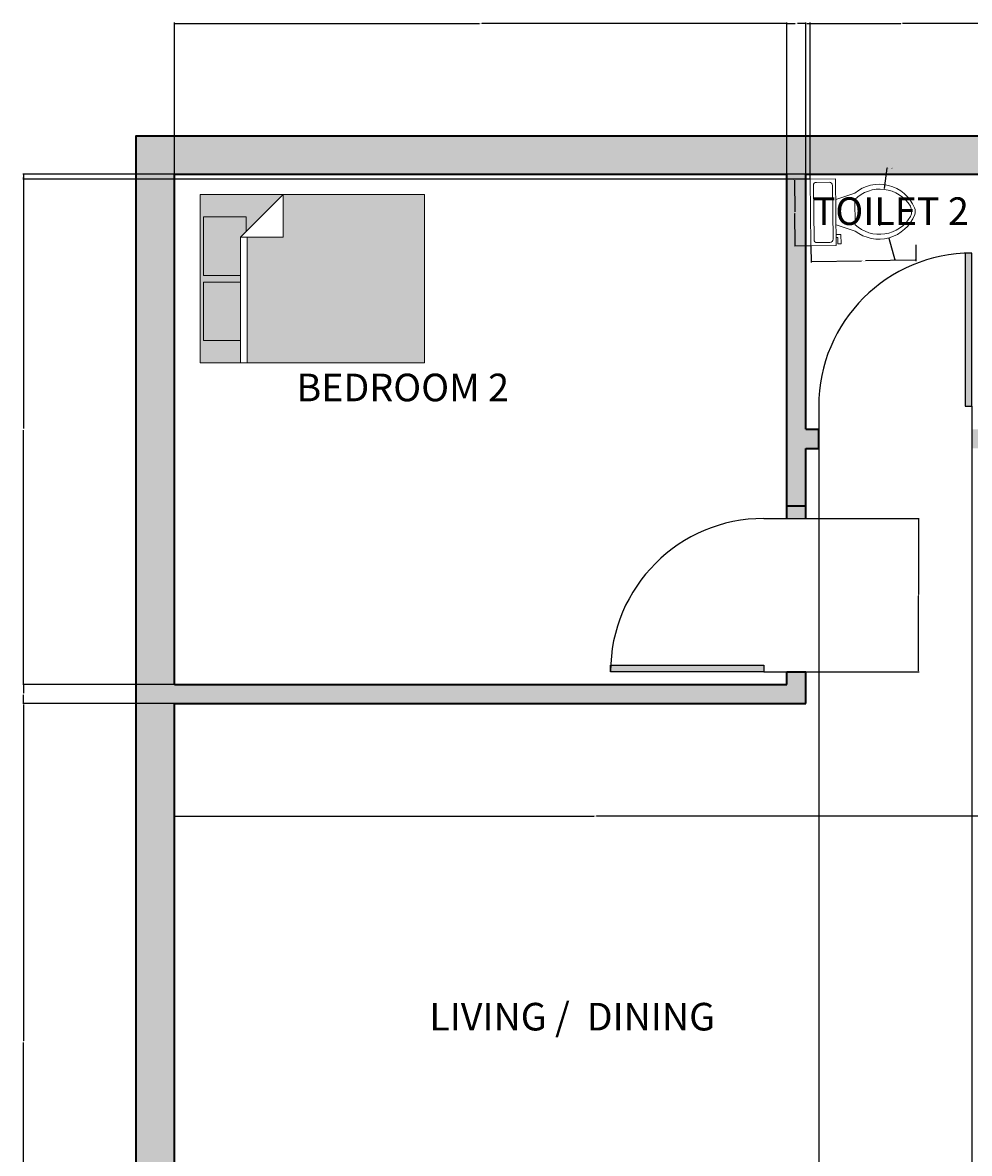
# Model space of a CAD drawing. Units: inches. Extents: x 1034 to 1730, y 674 to 1249.
# Tile 3 of 4: x 1316 to 1538, y 983 to 1249. Entities that reach past the tile are written whole.
import ezdxf

# ---------------------------------------------------------------- set-up
doc = ezdxf.new("R2010")
doc.units = ezdxf.units.IN
for name, color, linetype, lineweight in [('A-ANNO-DIMS', 2, 'Continuous', 18), ('A-AREA-IDEN', 7, 'Continuous', 18), ('A-DOOR', 4, 'Continuous', 25), ('A-FLOR-FIXT', 9, 'Continuous', 18), ('A-FURN', 9, 'Continuous', 18), ('A-FURN-PATT', 7, 'Continuous', 13), ('A-WALL', 7, 'Continuous', 35), ('A-WALL-PATT', 8, 'Continuous', 13)]:
    doc.layers.add(name, color=color, linetype=linetype, lineweight=lineweight)
doc.layers.add('A-DOOR-PATT', color=17, linetype='Continuous', lineweight=13, true_color=0x7b4636)
doc.styles.get("Standard").update_dxf_attribs({"font": 'arial.ttf'})
doc.dimstyles.get("Standard").update_dxf_attribs({"dimtxt": 0.18, "dimasz": 0.18, "dimexe": 0.18, "dimexo": 0.0625, "dimgap": 0.09, "dimtad": 0, "dimtih": 1, "dimtoh": 1, "dimdec": 4, "dimzin": 0, "dimdsep": 46, "dimtxsty": 'Standard', "dimcen": 0.09, "dimadec": 0, "dimazin": 0, "dimtfac": 1, "dimtdec": 4, "dimtofl": 0, "dimtmove": 0, "dimatfit": 3, "dimfxl": 1, "dimtolj": 1, "dimtzin": 0, "dimarcsym": 0})

# ---------------------------------------------------------------- blocks, each defined once
blk = doc.blocks.new('*U3')
for p, q in [((0, 0), (0, -6)), ((40, 0), (40, -6))]:
    blk.add_line(p, q)
blk.add_lwpolyline([(0, 0), (0, 40), (1.75, 40), (1.75, 0)], close=True)
blk.add_arc((0, 0), 40, 0, 90)
blk = doc.blocks.new('*U5')
for p, q in [((0, 0), (0, -6)), ((-40, 0), (-40, -6))]:
    blk.add_line(p, q)
blk.add_lwpolyline([(0, 0), (0, 40), (-1.75, 40), (-1.75, 0)], close=True)
blk.add_arc((0, 0), 40, 90, 180)
blk = doc.blocks.new('Bed - Queen')
for p, q in [((0, -80.00003), (0, 0)), ((0, 0), (59.99999, 0)), ((59.99999, 0), (59.99999, -80.00003)), ((7.99999, -1.2), (28.79998, -1.2)), ((7.99999, -14.4), (7.99999, -1.2)), ((28.79998, -1.2), (28.79998, -14.4)), ((31.19999, -1.2), (51.99999, -1.2)), ((31.19999, -14.4), (31.19999, -1.2)), ((51.99999, -1.2), (51.99999, -16.4)), ((0, -14.4), (44.8, -14.4)), ((59.99999, -29.6), (44.8, -14.4)), ((44.8, -14.4), (44.8, -29.6)), ((44.8, -16.8), (0, -16.8)), ((51.99999, -16.4), (46.79936, -16.4)), ((44.8, -29.6), (59.99999, -29.6)), ((59.99999, -80.00003), (0, -80.00003))]:
    blk.add_line(p, q)
blk = doc.blocks.new('Toilet - top')
for p, q in [((9.5, -6), (9.5, -2)), ((-10, -8.5), (-8, -8.5)), ((-10, -9.5), (-10, -8.5)), ((-7, -9.5), (-10, -9.5)), ((-8, -8.5), (-8, -8)), ((-7, -8), (-7, -9.5)), ((-4, -8), (-6, -14)), ((4, -8), (6, -14)), ((4, -14), (-4, -14))]:
    blk.add_line(p, q)
blk.add_lwpolyline([(10.5, -8), (10.5, 0), (-10.5, 0), (-10.5, -8)], close=True)
for points in [[(-9.5, -2), (-9.5, -6)], [(8.5, -1), (-8.5, -1)], [(-8.5, -7), (8.5, -7)]]:
    blk.add_lwpolyline(points)
for centre, radius, start, end in [((-8.62, -1.88), 0.884, 81.8699, 188.1301), ((8.62, -1.88), 0.884, 351.8699, 98.1301), ((-8.62, -6.12), 0.884, 171.8699, 278.1301), ((8.62, -6.12), 0.884, 261.8699, 8.1301), ((3.52, -21.58), 12.17, 141.4691, 247.9714), ((4.2, -21.82), 11.33, 136.3677, 238.9468), ((-3.52, -21.58), 12.17, 292.0284, 38.5307), ((-4.2, -21.82), 11.33, 301.053, 43.6321), ((0, -27.88), 4, 245.7318, 294.2682), ((0, -29), 4, 254.8605, 285.1395)]:
    blk.add_arc(centre, radius, start, end)
blk = doc.blocks.new('*D12')
at = {"layer": 'A-ANNO-DIMS', "color": 0, "lineweight": -2, "transparency": 16777216}
for p, q in [((1501.21, 1196.5), (1501.26, 1192.69)), ((1525.84, 1196.81), (1525.89, 1193)), ((1501.43, 1192.87), (1513.1, 1193.02)), ((1525.7, 1193.17), (1514.04, 1193.03))]:
    blk.add_line(p, q, dxfattribs=at)
at = {"layer": 'A-ANNO-DIMS', "color": 0, "transparency": 16777216}
for points in [[(1501.43, 1192.9), (1501.43, 1192.84), (1501.25, 1192.87)], [(1525.7, 1193.2), (1525.7, 1193.14), (1525.88, 1193.18)]]:
    blk.add_solid(points, dxfattribs=at)
at = {"layer": 'Defpoints', "color": 0, "transparency": 16777216}
for p in [(1501.21, 1196.57), (1525.84, 1196.87), (1501.25, 1192.87)]:
    blk.add_point(p, dxfattribs=at)
at = {"layer": 'A-ANNO-DIMS', "color": 0, "transparency": 16777216, "insert": (1513.57, 1193.02), "char_height": 0.18, "attachment_point": 5}
blk.add_mtext('\\A1;WC 25', dxfattribs=at)
blk = doc.blocks.new('*D13')
at = {"layer": 'A-ANNO-DIMS', "color": 0, "lineweight": -2, "transparency": 16777216}
for p, q in [((1500.95, 1212.22), (1497.14, 1212.17)), ((1497.32, 1211.99), (1497.41, 1204.53)), ((1497.51, 1196.7), (1497.42, 1204.16)), ((1501.15, 1196.56), (1497.33, 1196.52))]:
    blk.add_line(p, q, dxfattribs=at)
at = {"layer": 'A-ANNO-DIMS', "color": 0, "transparency": 16777216}
for points in [[(1497.35, 1211.99), (1497.29, 1211.99), (1497.32, 1212.17)], [(1497.54, 1196.7), (1497.48, 1196.7), (1497.51, 1196.52)]]:
    blk.add_solid(points, dxfattribs=at)
at = {"layer": 'Defpoints', "color": 0, "transparency": 16777216}
for p in [(1497.32, 1212.17), (1501.01, 1212.22), (1501.21, 1196.57)]:
    blk.add_point(p, dxfattribs=at)
at = {"layer": 'A-ANNO-DIMS', "color": 0, "transparency": 16777216, "insert": (1497.42, 1204.34), "char_height": 0.18, "attachment_point": 5}
blk.add_mtext('\\A1;16', dxfattribs=at)
blk = doc.blocks.new('*D17')
at = {"layer": 'A-ANNO-DIMS', "color": 0, "lineweight": -2, "transparency": 16777216}
for p, q in [((1351.53, 1213.49), (1351.53, 1249.06)), ((1351.71, 1248.88), (1423.25, 1248.88)), ((1495.35, 1248.88), (1423.81, 1248.88)), ((1495.53, 1213.49), (1495.53, 1249.06))]:
    blk.add_line(p, q, dxfattribs=at)
at = {"layer": 'A-ANNO-DIMS', "color": 0, "transparency": 16777216}
for points in [[(1351.71, 1248.91), (1351.71, 1248.85), (1351.53, 1248.88)], [(1495.35, 1248.91), (1495.35, 1248.85), (1495.53, 1248.88)]]:
    blk.add_solid(points, dxfattribs=at)
at = {"layer": 'Defpoints', "color": 0, "transparency": 16777216}
for p in [(1495.53, 1248.88), (1351.53, 1213.43), (1495.53, 1213.43)]:
    blk.add_point(p, dxfattribs=at)
at = {"layer": 'A-ANNO-DIMS', "color": 0, "transparency": 16777216, "insert": (1423.53, 1248.88), "char_height": 0.18, "attachment_point": 5}
blk.add_mtext('\\A1;144', dxfattribs=at)
blk = doc.blocks.new('*D19')
at = {"layer": 'A-ANNO-DIMS', "color": 0, "lineweight": -2, "transparency": 16777216}
for p, q in [((1351.47, 1213.43), (1315.9, 1213.43)), ((1316.08, 1213.25), (1316.08, 1153.61)), ((1316.08, 1093.61), (1316.08, 1153.24)), ((1351.47, 1093.43), (1315.9, 1093.43))]:
    blk.add_line(p, q, dxfattribs=at)
at = {"layer": 'A-ANNO-DIMS', "color": 0, "transparency": 16777216}
for points in [[(1316.05, 1213.25), (1316.11, 1213.25), (1316.08, 1213.43)], [(1316.05, 1093.61), (1316.11, 1093.61), (1316.08, 1093.43)]]:
    blk.add_solid(points, dxfattribs=at)
at = {"layer": 'Defpoints', "color": 0, "transparency": 16777216}
for p in [(1316.08, 1213.43), (1351.53, 1213.43), (1351.53, 1093.43)]:
    blk.add_point(p, dxfattribs=at)
at = {"layer": 'A-ANNO-DIMS', "color": 0, "transparency": 16777216, "insert": (1316.08, 1153.43), "char_height": 0.18, "attachment_point": 5}
blk.add_mtext('\\A1;120', dxfattribs=at)
blk = doc.blocks.new('*D20')
at = {"layer": 'A-ANNO-DIMS', "color": 0, "lineweight": -2, "transparency": 16777216}
for p, q in [((1351.47, 1088.93), (1315.9, 1088.93)), ((1316.08, 1088.75), (1316.08, 1009.61)), ((1316.08, 930.11), (1316.08, 1009.24)), ((1351.47, 929.93), (1315.9, 929.93))]:
    blk.add_line(p, q, dxfattribs=at)
at = {"layer": 'A-ANNO-DIMS', "color": 0, "transparency": 16777216}
for points in [[(1316.05, 1088.75), (1316.11, 1088.75), (1316.08, 1088.93)], [(1316.05, 930.11), (1316.11, 930.11), (1316.08, 929.93)]]:
    blk.add_solid(points, dxfattribs=at)
at = {"layer": 'Defpoints', "color": 0, "transparency": 16777216}
for p in [(1316.08, 1088.93), (1351.53, 1088.93), (1351.53, 929.93)]:
    blk.add_point(p, dxfattribs=at)
at = {"layer": 'A-ANNO-DIMS', "color": 0, "transparency": 16777216, "insert": (1316.08, 1009.43), "char_height": 0.18, "attachment_point": 5}
blk.add_mtext('\\A1;159', dxfattribs=at)
blk = doc.blocks.new('*D26')
at = {"layer": 'A-ANNO-DIMS', "color": 0, "lineweight": -2, "transparency": 16777216}
for p, q in [((1500.03, 1213.49), (1500.03, 1249.06)), ((1500.21, 1248.88), (1522.31, 1248.88)), ((1544.85, 1248.88), (1522.75, 1248.88)), ((1545.03, 1213.49), (1545.03, 1249.06))]:
    blk.add_line(p, q, dxfattribs=at)
at = {"layer": 'A-ANNO-DIMS', "color": 0, "transparency": 16777216}
for points in [[(1500.21, 1248.91), (1500.21, 1248.85), (1500.03, 1248.88)], [(1544.85, 1248.91), (1544.85, 1248.85), (1545.03, 1248.88)]]:
    blk.add_solid(points, dxfattribs=at)
at = {"layer": 'Defpoints', "color": 0, "transparency": 16777216}
for p in [(1545.03, 1248.88), (1500.03, 1213.43), (1545.03, 1213.43)]:
    blk.add_point(p, dxfattribs=at)
at = {"layer": 'A-ANNO-DIMS', "color": 0, "transparency": 16777216, "insert": (1522.53, 1248.88), "char_height": 0.18, "attachment_point": 5}
blk.add_mtext('\\A1;45', dxfattribs=at)
blk = doc.blocks.new('*D28')
at = {"layer": 'A-ANNO-DIMS', "color": 0, "lineweight": -2, "transparency": 16777216}
for p, q in [((1503.03, 1153.36), (1503.03, 673.53)), ((1539.03, 1153.36), (1539.03, 673.53)), ((1503.21, 673.71), (1520.81, 673.71)), ((1538.85, 673.71), (1521.25, 673.71))]:
    blk.add_line(p, q, dxfattribs=at)
at = {"layer": 'A-ANNO-DIMS', "color": 0, "transparency": 16777216}
for points in [[(1503.21, 673.74), (1503.21, 673.68), (1503.03, 673.71)], [(1538.85, 673.74), (1538.85, 673.68), (1539.03, 673.71)]]:
    blk.add_solid(points, dxfattribs=at)
at = {"layer": 'Defpoints', "color": 0, "transparency": 16777216}
for p in [(1503.03, 1153.43), (1539.03, 1153.43), (1539.03, 673.71)]:
    blk.add_point(p, dxfattribs=at)
at = {"layer": 'A-ANNO-DIMS', "color": 0, "transparency": 16777216, "insert": (1521.03, 673.71), "char_height": 0.18, "attachment_point": 5}
blk.add_mtext('\\A1;36', dxfattribs=at)
blk = doc.blocks.new('*D43')
at = {"layer": 'A-ANNO-DIMS', "color": 0, "lineweight": -2, "transparency": 16777216}
for p, q in [((1495.53, 1213.49), (1495.53, 1249.06)), ((1495.71, 1248.88), (1497.52, 1248.88)), ((1499.85, 1248.88), (1498.04, 1248.88)), ((1500.03, 1213.49), (1500.03, 1249.06))]:
    blk.add_line(p, q, dxfattribs=at)
at = {"layer": 'A-ANNO-DIMS', "color": 0, "transparency": 16777216}
for points in [[(1495.71, 1248.91), (1495.71, 1248.85), (1495.53, 1248.88)], [(1499.85, 1248.91), (1499.85, 1248.85), (1500.03, 1248.88)]]:
    blk.add_solid(points, dxfattribs=at)
at = {"layer": 'Defpoints', "color": 0, "transparency": 16777216}
for p in [(1500.03, 1248.88), (1495.53, 1213.43), (1500.03, 1213.43)]:
    blk.add_point(p, dxfattribs=at)
at = {"layer": 'A-ANNO-DIMS', "color": 0, "transparency": 16777216, "insert": (1497.78, 1248.88), "char_height": 0.18, "attachment_point": 5}
blk.add_mtext('\\A1;4.5', dxfattribs=at)
blk = doc.blocks.new('*D45')
at = {"layer": 'A-ANNO-DIMS', "color": 0, "lineweight": -2, "transparency": 16777216}
for p, q in [((1500.09, 1132.43), (1526.66, 1132.43)), ((1526.48, 1132.25), (1526.48, 1114.61)), ((1526.48, 1096.61), (1526.48, 1114.24)), ((1500.09, 1096.43), (1526.66, 1096.43))]:
    blk.add_line(p, q, dxfattribs=at)
at = {"layer": 'A-ANNO-DIMS', "color": 0, "transparency": 16777216}
for points in [[(1526.45, 1132.25), (1526.51, 1132.25), (1526.48, 1132.43)], [(1526.45, 1096.61), (1526.51, 1096.61), (1526.48, 1096.43)]]:
    blk.add_solid(points, dxfattribs=at)
at = {"layer": 'Defpoints', "color": 0, "transparency": 16777216}
for p in [(1500.03, 1132.43), (1500.03, 1096.43), (1526.48, 1096.43)]:
    blk.add_point(p, dxfattribs=at)
at = {"layer": 'A-ANNO-DIMS', "color": 0, "transparency": 16777216, "insert": (1526.48, 1114.43), "char_height": 0.18, "attachment_point": 5}
blk.add_mtext('\\A1;36', dxfattribs=at)
blk = doc.blocks.new('*D46')
at = {"layer": 'A-ANNO-DIMS', "color": 0, "lineweight": -2, "transparency": 16777216}
for p, q in [((1351.53, 1088.86), (1351.53, 1062.3)), ((1549.53, 1088.86), (1549.53, 1062.3)), ((1351.71, 1062.48), (1450.25, 1062.48)), ((1549.35, 1062.48), (1450.81, 1062.48))]:
    blk.add_line(p, q, dxfattribs=at)
at = {"layer": 'A-ANNO-DIMS', "color": 0, "transparency": 16777216}
for points in [[(1351.71, 1062.51), (1351.71, 1062.45), (1351.53, 1062.48)], [(1549.35, 1062.51), (1549.35, 1062.45), (1549.53, 1062.48)]]:
    blk.add_solid(points, dxfattribs=at)
at = {"layer": 'Defpoints', "color": 0, "transparency": 16777216}
for p in [(1351.53, 1088.93), (1549.53, 1088.93), (1351.53, 1062.48)]:
    blk.add_point(p, dxfattribs=at)
at = {"layer": 'A-ANNO-DIMS', "color": 0, "transparency": 16777216, "insert": (1450.53, 1062.48), "char_height": 0.18, "attachment_point": 5}
blk.add_mtext('\\A1;198', dxfattribs=at)
blk = doc.blocks.new('*D51')
at = {"layer": 'A-ANNO-DIMS', "color": 0, "lineweight": -2, "transparency": 16777216}
for p, q in [((1499.848848, 1248.87622), (1499.668848, 1248.87622)), ((1500.028848, 1213.48872), (1500.028848, 1249.05622)), ((1501.01344, 1212.278928), (1501.01344, 1249.05622)), ((1501.19344, 1248.87622), (1501.37344, 1248.87622))]:
    blk.add_line(p, q, dxfattribs=at)
at = {"layer": 'A-ANNO-DIMS', "color": 0, "transparency": 16777216}
for points in [[(1499.848848, 1248.90622), (1499.848848, 1248.84622), (1500.028848, 1248.87622)], [(1501.19344, 1248.90622), (1501.19344, 1248.84622), (1501.01344, 1248.87622)]]:
    blk.add_solid(points, dxfattribs=at)
at = {"layer": 'Defpoints', "color": 0, "transparency": 16777216}
for p in [(1500.028848, 1248.87622), (1500.028848, 1213.42622), (1501.01344, 1212.216428)]:
    blk.add_point(p, dxfattribs=at)
at = {"layer": 'A-ANNO-DIMS', "color": 0, "transparency": 16777216, "insert": (1500.521144, 1248.87622), "char_height": 0.18, "attachment_point": 5}
blk.add_mtext('\\A1;0.98', dxfattribs=at)
blk = doc.blocks.new('*D52')
at = {"layer": 'A-ANNO-DIMS', "color": 0, "lineweight": -2, "transparency": 16777216}
for p, q in [((1499.97, 1213.43), (1315.9, 1213.43)), ((1316.08, 1213.25), (1316.08, 1213)), ((1316.08, 1212.4), (1316.08, 1212.64)), ((1500.95, 1212.22), (1315.9, 1212.22))]:
    blk.add_line(p, q, dxfattribs=at)
at = {"layer": 'A-ANNO-DIMS', "color": 0, "transparency": 16777216}
for points in [[(1316.05, 1213.25), (1316.11, 1213.25), (1316.08, 1213.43)], [(1316.05, 1212.4), (1316.11, 1212.4), (1316.08, 1212.22)]]:
    blk.add_solid(points, dxfattribs=at)
at = {"layer": 'Defpoints', "color": 0, "transparency": 16777216}
for p in [(1316.08, 1213.43), (1500.03, 1213.43), (1501.01, 1212.22)]:
    blk.add_point(p, dxfattribs=at)
at = {"layer": 'A-ANNO-DIMS', "color": 0, "transparency": 16777216, "insert": (1316.08, 1212.82), "char_height": 0.18, "attachment_point": 5}
blk.add_mtext('\\A1;1.21', dxfattribs=at)
blk = doc.blocks.new('*D53')
at = {"layer": 'A-ANNO-DIMS', "color": 0, "lineweight": -2, "transparency": 16777216}
for p, q in [((1351.47, 1093.43), (1315.9, 1093.43)), ((1316.08, 1093.25), (1316.08, 1091.36)), ((1316.08, 1089.11), (1316.08, 1090.99)), ((1351.47, 1088.93), (1315.9, 1088.93))]:
    blk.add_line(p, q, dxfattribs=at)
at = {"layer": 'A-ANNO-DIMS', "color": 0, "transparency": 16777216}
for points in [[(1316.05, 1093.25), (1316.11, 1093.25), (1316.08, 1093.43)], [(1316.05, 1089.11), (1316.11, 1089.11), (1316.08, 1088.93)]]:
    blk.add_solid(points, dxfattribs=at)
at = {"layer": 'Defpoints', "color": 0, "transparency": 16777216}
for p in [(1316.08, 1093.43), (1351.53, 1093.43), (1351.53, 1088.93)]:
    blk.add_point(p, dxfattribs=at)
at = {"layer": 'A-ANNO-DIMS', "color": 0, "transparency": 16777216, "insert": (1316.08, 1091.18), "char_height": 0.18, "attachment_point": 5}
blk.add_mtext('\\A1;4.5', dxfattribs=at)
blk = doc.blocks.new('*D57')
at = {"layer": 'A-ANNO-DIMS', "color": 0, "lineweight": -2, "transparency": 16777216}
for p, q in [((1517.07, 1207.21), (1517.25, 1207.21)), ((1517.16, 1207.12), (1517.16, 1207.3)), ((1521.02, 1193.22), (1519.62, 1198.3)), ((1521.2, 1193.22), (1521.02, 1193.22))]:
    blk.add_line(p, q, dxfattribs=at)
at = {"layer": 'A-ANNO-DIMS', "color": 0, "transparency": 16777216}
blk.add_solid([(1519.65, 1198.3), (1519.59, 1198.29), (1519.57, 1198.47)], dxfattribs=at)
at = {"layer": 'Defpoints', "color": 0, "transparency": 16777216}
for p in [(1517.16, 1207.21), (1519.57, 1198.47)]:
    blk.add_point(p, dxfattribs=at)
at = {"layer": 'A-ANNO-DIMS', "color": 0, "transparency": 16777216, "insert": (1521.81, 1193.22), "char_height": 0.18, "attachment_point": 5}
blk.add_mtext('\\A1;2X R9.07', dxfattribs=at)
blk = doc.blocks.new('*D58')
at = {"layer": 'A-ANNO-DIMS', "color": 0, "lineweight": -2, "transparency": 16777216}
for p, q in [((1519.04, 1214.87), (1518.45, 1210.02)), ((1519.22, 1214.87), (1519.04, 1214.87)), ((1517.32, 1201.46), (1517.5, 1201.46)), ((1517.41, 1201.37), (1517.41, 1201.55))]:
    blk.add_line(p, q, dxfattribs=at)
at = {"layer": 'A-ANNO-DIMS', "color": 0, "transparency": 16777216}
blk.add_solid([(1518.42, 1210.03), (1518.48, 1210.02), (1518.43, 1209.84)], dxfattribs=at)
at = {"layer": 'Defpoints', "color": 0, "transparency": 16777216}
for p in [(1518.43, 1209.84), (1517.41, 1201.46)]:
    blk.add_point(p, dxfattribs=at)
at = {"layer": 'A-ANNO-DIMS', "color": 0, "transparency": 16777216, "insert": (1519.9, 1214.87), "char_height": 0.18, "attachment_point": 5}
blk.add_mtext('\\A1;2X R8.444', dxfattribs=at)

msp = doc.modelspace()

# ---------------------------------------------------------------- hatches: boundary and pattern name
at = {"layer": 'A-DOOR-PATT'}
h = msp.add_hatch(color=256, dxfattribs=at)
h.dxf.hatch_style = 1
h.paths.add_polyline_path([(1490.123, 922.4262), (1454.0839, 922.4262, 0.01094143), (1454.1184, 920.8495), (1490.123, 920.8495)])
h.paths.add_polyline_path([(1540.7238, 871.4262), (1504.6847, 871.4262), (1504.6847, 869.8495), (1540.6893, 869.8495, 0.01094143)])
h.paths.add_polyline_path([(1503.0288, 874.4262), (1495.5288, 874.4262), (1495.5288, 871.4262), (1503.0288, 871.4262)])
h.paths.add_polyline_path([(1503.0288, 835.3871), (1499.2788, 835.3871), (1495.5288, 835.4262), (1495.5288, 832.4262), (1503.0288, 832.4262)])
h.paths.add_polyline_path([(1564.6056, 873.3367, 0.01094143), (1563.0288, 873.3712), (1563.0288, 837.3321), (1564.6056, 837.3321)])
h.paths.add_polyline_path([(1602.0288, 831.9262), (1599.0288, 831.9262), (1599.0288, 828.9262), (1602.0288, 828.9262)])
h.paths.add_polyline_path([(1648.5288, 988.4262), (1645.5288, 988.4262), (1645.5288, 985.4262), (1648.5288, 985.4262)])
h.paths.add_polyline_path([(1689.9738, 989.9638), (1653.9347, 989.9638), (1653.9347, 988.3871), (1689.9738, 988.3871)])
h.paths.add_polyline_path([(1648.5288, 1027.4262), (1645.5288, 1027.4262), (1645.5288, 1024.4262), (1648.5288, 1024.4262)])
h.paths.add_polyline_path([(1590.9393, 1097.9638), (1554.9347, 1097.9638), (1554.9347, 1096.3871), (1590.9738, 1096.3871, 0.01094143)])
h.paths.add_polyline_path([(1549.5288, 1135.4262), (1545.0288, 1135.4262), (1545.0288, 1132.4262), (1549.5288, 1132.4262)])
h.paths.add_polyline_path([(1500.0288, 1135.4262), (1495.5288, 1135.4262), (1495.5288, 1132.4262), (1500.0288, 1132.4262)])
h.paths.add_polyline_path([(1490.123, 1098.0029), (1454.0839, 1098.0029), (1454.0839, 1096.4262), (1490.123, 1096.4262)])
h.paths.add_polyline_path([(1539.068, 1194.8712, 0.01094143), (1537.4912, 1194.8367), (1537.4912, 1158.8321), (1539.068, 1158.8321)])
at = {"layer": 'A-FURN-PATT'}
h = msp.add_hatch(color=256, dxfattribs=at)
h.dxf.hatch_style = 1
h.paths.add_polyline_path([(1414.278, 838.2731), (1381.0078, 838.2731), (1381.0078, 828.2392), (1372.5582, 828.2392), (1372.5582, 798.6657), (1414.278, 798.6657)])
h.paths.add_polyline_path([(1370.9739, 828.2392), (1372.2941, 829.5594), (1372.2941, 832.9921), (1362.2603, 832.9921), (1362.2603, 819.2615), (1370.9739, 819.2615)], flags=17)
h.paths.add_polyline_path([(1370.9739, 817.6772), (1362.2603, 817.6772), (1362.2603, 803.9467), (1370.9739, 803.9467)], flags=17)
h.paths.add_polyline_path([(1367.0568, 1198.6055), (1368.377, 1199.9257), (1368.377, 1203.3584), (1358.3431, 1203.3584), (1358.3431, 1189.6278), (1367.0568, 1189.6278)], flags=17)
h.paths.add_polyline_path([(1367.0568, 1188.0435), (1358.3431, 1188.0435), (1358.3431, 1174.3129), (1367.0568, 1174.3129)], flags=17)
h.paths.add_polyline_path([(1410.3609, 1208.6394), (1377.0906, 1208.6394), (1377.0906, 1198.6055), (1368.6411, 1198.6055), (1368.6411, 1169.032), (1410.3609, 1169.032)])
h.paths.add_polyline_path([(1678.2824, 1203.4604), (1636.5626, 1203.4604), (1636.5626, 1163.853), (1669.8329, 1163.853), (1669.8329, 1173.8868), (1678.2824, 1173.8868)])
h.paths.add_polyline_path([(1688.5804, 1182.8645), (1679.8667, 1182.8645), (1679.8667, 1173.8868), (1678.5465, 1172.5666), (1678.5465, 1169.1339), (1688.5804, 1169.1339)], flags=17)
h.paths.add_polyline_path([(1367.0568, 1174.3129), (1358.3431, 1174.3129), (1358.3431, 1188.0435), (1367.0568, 1188.0435), (1367.0568, 1189.6278), (1358.3431, 1189.6278), (1358.3431, 1203.3584), (1368.377, 1203.3584), (1368.377, 1199.9257), (1377.0906, 1208.6394), (1357.551, 1208.6394), (1357.551, 1169.032), (1367.0568, 1169.032)])
h.paths.add_polyline_path([(1688.5804, 1198.1794), (1679.8667, 1198.1794), (1679.8667, 1184.4488), (1688.5804, 1184.4488)], flags=17)
h.paths.add_polyline_path([(1689.3725, 1203.4604), (1679.8667, 1203.4604), (1679.8667, 1198.1794), (1688.5804, 1198.1794), (1688.5804, 1184.4488), (1679.8667, 1184.4488), (1679.8667, 1182.8645), (1688.5804, 1182.8645), (1688.5804, 1169.1339), (1678.5465, 1169.1339), (1678.5465, 1172.5666), (1669.8329, 1163.853), (1689.3725, 1163.853)])
h.paths.add_polyline_path([(1370.9739, 803.9467), (1362.2603, 803.9467), (1362.2603, 817.6772), (1370.9739, 817.6772), (1370.9739, 819.2615), (1362.2603, 819.2615), (1362.2603, 832.9921), (1372.2941, 832.9921), (1372.2941, 829.5594), (1381.0078, 838.2731), (1361.4681, 838.2731), (1361.4681, 798.6657), (1370.9739, 798.6657)])
h.paths.add_polyline_path([(1586.4252, 1162.5974), (1646.7165, 1162.5974), (1646.7165, 1172.6784), (1586.4252, 1172.6784)], flags=9)
h.paths.add_polyline_path([(1574.2942, 863.9077), (1611.4062, 863.9077), (1611.4062, 873.9821), (1574.2942, 873.9821)], flags=9)
h.paths.add_polyline_path([(1502.8652, 818.6383), (1550.5629, 818.6383), (1550.5629, 828.7127), (1502.8652, 828.7127)], flags=9)
h.paths.add_polyline_path([(1367.7365, 861.2327), (1425.5064, 861.2327), (1425.5064, 871.3071), (1367.7365, 871.3071)], flags=9)
h.paths.add_polyline_path([(1409.7909, 1010.2859), (1487.2071, 1010.2859), (1487.2071, 1020.3537), (1409.7909, 1020.3537)], flags=9)
h.paths.add_polyline_path([(1499.9637, 1199.6865), (1545.1423, 1199.6865), (1545.1423, 1209.7608), (1499.9637, 1209.7608)], flags=9)
h.paths.add_polyline_path([(1378.5639, 1158.2313), (1436.3338, 1158.2313), (1436.3338, 1168.3057), (1378.5639, 1168.3057)], flags=9)
at = {"layer": 'A-WALL-PATT'}
h = msp.add_hatch(color=256, dxfattribs=at)
h.dxf.hatch_style = 1
h.paths.add_polyline_path([(1351.5288, 1213.4262), (1495.5288, 1213.4262), (1495.5288, 1135.4262), (1500.0288, 1135.4262), (1500.0288, 1148.9262), (1503.0288, 1148.9262), (1503.0288, 1153.4262), (1500.0288, 1153.4262), (1500.0288, 1213.4262), (1545.0288, 1213.4262), (1545.0288, 1153.4262), (1539.0288, 1153.4262), (1539.0288, 1148.9262), (1545.0288, 1148.9262), (1545.0288, 1135.4262), (1549.5288, 1135.4262), (1549.5288, 1213.4262), (1693.5288, 1213.4262), (1693.5288, 1093.4262), (1549.5288, 1093.4262), (1549.5288, 1096.4262), (1545.0288, 1096.4262), (1545.0288, 1088.9262), (1549.5288, 1088.9262), (1549.5288, 1064.9262), (1552.5288, 1064.9262), (1552.5288, 1088.9262), (1645.5288, 1088.9262), (1645.5288, 1027.4262), (1648.5288, 1027.4262), (1648.5288, 1088.9262), (1693.5288, 1088.9262), (1693.5288, 985.4262), (1552.5288, 985.4262), (1552.5288, 1004.9262), (1549.5288, 1004.9262), (1549.5288, 980.9262), (1620.0288, 980.9262), (1620.0288, 831.9262), (1602.0288, 831.9262), (1602.0288, 828.9262), (1624.5288, 828.9262), (1624.5288, 980.9262), (1693.5288, 980.9262), (1693.5288, 742.4262), (1702.5288, 742.4262), (1702.5288, 1222.4262), (1342.5288, 1222.4262), (1342.5288, 742.4262), (1620.0288, 742.4262), (1620.0288, 751.4262), (1351.5288, 751.4262), (1351.5288, 788.9262), (1560.0288, 788.9262), (1560.0288, 828.9262), (1563.0288, 828.9262), (1563.0288, 831.9262), (1560.0288, 831.9262), (1560.0288, 886.4262), (1500.0288, 886.4262), (1495.5288, 886.4262), (1495.5288, 874.4262), (1503.0288, 874.4262), (1503.0288, 883.4262), (1557.0288, 883.4262), (1557.0288, 791.9262), (1503.0288, 791.9262), (1503.0288, 832.4262), (1495.5288, 832.4262), (1495.5288, 793.4262), (1351.5288, 793.4262), (1351.5288, 925.4262), (1495.5288, 925.4262), (1495.5288, 922.4262), (1500.0288, 922.4262), (1500.0288, 929.9262), (1351.5288, 929.9262), (1351.5288, 1088.9262), (1500.0288, 1088.9262), (1500.0288, 1096.4262), (1495.5288, 1096.4262), (1495.5288, 1093.4262), (1351.5288, 1093.4262)])

# ---------------------------------------------------------------- linework, layer by layer
at = {"layer": 'A-DOOR'}
msp.add_line((1495.5288, 1132.4262), (1500.0288, 1132.4262), dxfattribs=at)
at = {"layer": 'A-WALL'}
for p, q in [((1351.5288, 1213.4262), (1495.5288, 1213.4262)), ((1351.5288, 1093.4262), (1351.5288, 1213.4262)), ((1495.5288, 1132.4262), (1495.5288, 1213.4262)), ((1500.0288, 1153.4262), (1500.0288, 1213.4262)), ((1500.0288, 1213.4262), (1545.0288, 1213.4262)), ((1500.0288, 1153.4262), (1503.0288, 1153.4262)), ((1503.0288, 1148.9262), (1503.0288, 1153.4262)), ((1500.0288, 1148.9262), (1503.0288, 1148.9262)), ((1500.0288, 1132.4262), (1500.0288, 1148.9262)), ((1495.5288, 1135.4262), (1500.0288, 1135.4262)), ((1495.5288, 1093.4262), (1495.5288, 1096.4262)), ((1495.5288, 1096.4262), (1500.0288, 1096.4262)), ((1500.0288, 1088.9262), (1500.0288, 1096.4262)), ((1351.5288, 1093.4262), (1495.5288, 1093.4262)), ((1351.5288, 1088.9262), (1500.0288, 1088.9262)), ((1351.5288, 929.9262), (1351.5288, 1088.9262))]:
    msp.add_line(p, q, dxfattribs=at)
msp.add_lwpolyline([(1620.0288, 742.4262), (1342.5288, 742.4262), (1342.5288, 1222.4262), (1702.5288, 1222.4262), (1702.5288, 742.4262), (1693.5288, 742.4262)], dxfattribs=at)

# ---------------------------------------------------------------- block references
at = {"layer": 'A-DOOR', "xscale": 0.9009776753840846, "yscale": 0.9009776753840846, "zscale": 0.9009776753840846}
msp.add_blockref('*U5', (1539.068, 1158.8321), dxfattribs=at)
at = {"layer": 'A-DOOR', "xscale": 0.9009776753840846, "yscale": 0.9009776753840846, "zscale": 0.9009776753840846, "rotation": 90}
msp.add_blockref('*U3', (1490.123, 1096.4262), dxfattribs=at)
at = {"layer": 'A-FLOR-FIXT', "xscale": 0.7453567138886678, "yscale": 0.7453567138886678, "zscale": 0.7453567138886678, "rotation": 90.71118291069774}
msp.add_blockref('Toilet - top', (1501.1106, 1204.3908), dxfattribs=at)
at = {"layer": 'A-FURN', "xscale": 0.6601233642522663, "yscale": 0.6601233642522663, "zscale": 0.6601233642522663, "rotation": 90}
msp.add_blockref('Bed - Queen', (1357.551, 1169.032), dxfattribs=at)

# ---------------------------------------------------------------- texts
at = {"layer": 'A-AREA-IDEN'}
for s, height, p in [('TOILET 2 ', 6.49045, (1501.6428, 1201.4762)), ('BEDROOM 2', 6.49045, (1380.243, 1160.0211)), ('LIVING /  DINING ', 6.490455, (1411.4689, 1012.0746))]:
    msp.add_text(s, height=height, dxfattribs=at).set_placement(p)

# ---------------------------------------------------------------- dimensions: what is measured, and where the dimension line sits
at = {"layer": 'A-ANNO-DIMS'}
for base, p1, p2, override, picture, middle in [((1495.5288, 1248.8762), (1351.5288, 1213.4262), (1495.5288, 1213.4262), {"dimdec": 0, "dimlfac": 1, "dimrnd": 0, "dimzin": 0, "dimdsep": 46, "dimlunit": 2}, '*D17', (1423.5288, 1248.8762)), ((1500.0288, 1248.8762), (1495.5288, 1213.4262), (1500.0288, 1213.4262), {"dimdec": 1, "dimlfac": 1, "dimrnd": 0, "dimzin": 0, "dimdsep": 46, "dimlunit": 2}, '*D43', (1497.7788, 1248.8762)), ((1500.0288, 1248.8762), (1501.0134, 1212.2164), (1500.0288, 1213.4262), {"dimdec": 2, "dimlfac": 1, "dimrnd": 0, "dimzin": 0, "dimdsep": 46, "dimlunit": 2}, '*D51', (1500.5211, 1248.8762)), ((1545.0288, 1248.8762), (1500.0288, 1213.4262), (1545.0288, 1213.4262), {"dimdec": 0, "dimlfac": 1, "dimrnd": 0, "dimzin": 0, "dimdsep": 46, "dimlunit": 2}, '*D26', (1522.5288, 1248.8762)), ((1539.0288, 673.7132), (1503.0288, 1153.4262), (1539.0288, 1153.4262), {"dimdec": 0, "dimlfac": 1, "dimrnd": 0, "dimzin": 0, "dimdsep": 46, "dimlunit": 2}, '*D28', (1521.0288, 673.7132))]:
    dim = msp.add_linear_dim(base=base, p1=p1, p2=p2, dimstyle='Standard', override=override, dxfattribs=at)
    dim.commit()
    dim.dimension.update_dxf_attribs({"geometry": picture, "text_midpoint": middle})
for center, mpoint, override, picture, middle in [((1517.4099, 1201.4625), (1518.431, 1209.8448), {"dimdec": 3, "dimlfac": 1, "dimrnd": 0, "dimzin": 0, "dimdsep": 46, "dimlunit": 2}, '*D58', (1519.898, 1214.8742)), ((1517.1619, 1207.2136), (1519.575, 1198.4702), {"dimdec": 2, "dimlfac": 1, "dimrnd": 0, "dimzin": 0, "dimdsep": 46, "dimlunit": 2}, '*D57', (1521.8076, 1193.2241))]:
    dim = msp.add_radius_dim(center=center, mpoint=mpoint, text='2X <>', dimstyle='Standard', override=override, dxfattribs=at)
    dim.commit()
    dim.dimension.update_dxf_attribs({"geometry": picture, "text_midpoint": middle, "dimtype": 164})
for base, p1, p2, angle, override, picture, middle in [((1316.0788, 1213.4262), (1501.0134, 1212.2164), (1500.0288, 1213.4262), 90, {"dimdec": 2, "dimlfac": 1, "dimrnd": 0, "dimzin": 0, "dimdsep": 46, "dimlunit": 2}, '*D52', (1316.0788, 1212.8213)), ((1316.0788, 1213.4262), (1351.5288, 1093.4262), (1351.5288, 1213.4262), 90, {"dimdec": 0, "dimlfac": 1, "dimrnd": 0, "dimzin": 0, "dimdsep": 46, "dimlunit": 2}, '*D19', (1316.0788, 1153.4262)), ((1497.319, 1212.1706), (1501.2077, 1196.5651), (1501.0134, 1212.2164), 90.711183, {"dimdec": 0, "dimlfac": 1, "dimrnd": 0, "dimzin": 0, "dimdsep": 46, "dimlunit": 2}, '*D13', (1497.4162, 1204.3449)), ((1526.4788, 1096.4262), (1500.0288, 1132.4262), (1500.0288, 1096.4262), 270, {"dimdec": 0, "dimlfac": 1, "dimrnd": 0, "dimzin": 0, "dimdsep": 46, "dimlunit": 2}, '*D45', (1526.4788, 1114.4262)), ((1316.0788, 1093.4262), (1351.5288, 1088.9262), (1351.5288, 1093.4262), 90, {"dimdec": 1, "dimlfac": 1, "dimrnd": 0, "dimzin": 0, "dimdsep": 46, "dimlunit": 2}, '*D53', (1316.0788, 1091.1762)), ((1316.0788, 1088.9262), (1351.5288, 929.9262), (1351.5288, 1088.9262), 90, {"dimdec": 0, "dimlfac": 1, "dimrnd": 0, "dimzin": 0, "dimdsep": 46, "dimlunit": 2}, '*D20', (1316.0788, 1009.4262)), ((1351.5288, 1062.4762), (1549.5288, 1088.9262), (1351.5288, 1088.9262), 180, {"dimdec": 0, "dimlfac": 1, "dimrnd": 0, "dimzin": 0, "dimdsep": 46, "dimlunit": 2}, '*D46', (1450.5288, 1062.4762))]:
    dim = msp.add_linear_dim(base=base, p1=p1, p2=p2, angle=angle, dimstyle='Standard', override=override, dxfattribs=at)
    dim.commit()
    dim.dimension.update_dxf_attribs({"geometry": picture, "text_midpoint": middle})
dim = msp.add_linear_dim(base=(1501.2536, 1192.8707), p1=(1525.8371, 1196.8709), p2=(1501.2077, 1196.5651), angle=180.711183, text='WC <>', dimstyle='Standard', override={"dimdec": 0, "dimlfac": 1, "dimrnd": 0, "dimzin": 0, "dimdsep": 46, "dimlunit": 2}, dxfattribs=at)
dim.commit()
dim.dimension.update_dxf_attribs({"geometry": '*D12', "text_midpoint": (1513.5683, 1193.0236)})

doc.saveas('drawing.dxf')
